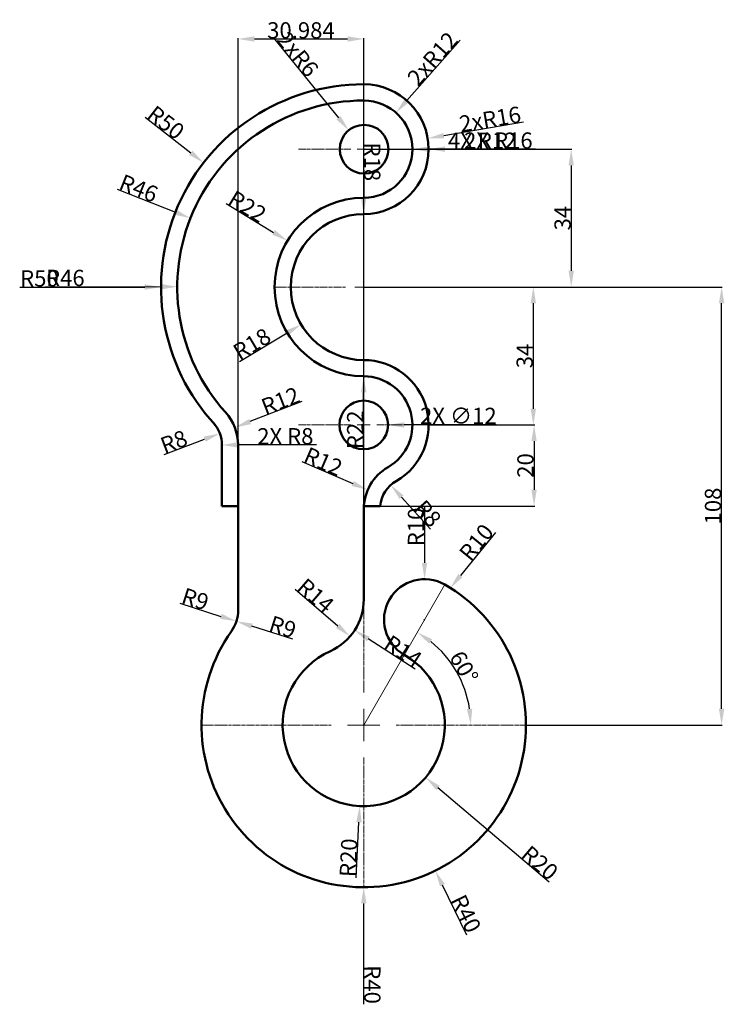
# Model space of a CAD drawing. Units: millimetres. Extents: x 64 to 238, y 47 to 290.
import ezdxf

# ---------------------------------------------------------------- set-up
doc = ezdxf.new("R2010")
doc.units = ezdxf.units.MM
doc.header["$MEASUREMENT"] = 0
doc.linetypes.add('CENTER2', pattern=[1.125, 0.75, -0.125, 0.125, -0.125])
for name, color, linetype, lineweight in [('M-CNTR', 4, 'CENTER2', 18), ('M-CONS', 8, 'Continuous', 13), ('M-DIMS', 2, 'Continuous', 25), ('M-OUTL', 7, 'Continuous', 50)]:
    doc.layers.add(name, color=color, linetype=linetype, lineweight=lineweight)
doc.styles.get("Standard").update_dxf_attribs({"font": 'arial.ttf'})
doc.dimstyles.get("Standard").update_dxf_attribs({"dimtxt": 4, "dimasz": 4, "dimexe": 0.18, "dimexo": 0.0625, "dimgap": 0.09, "dimtad": 1, "dimdec": 0, "dimzin": 0, "dimdsep": 46, "dimtxsty": 'Standard', "dimcen": 0.09, "dimclre": 251, "dimadec": 0, "dimazin": 0, "dimtfac": 1, "dimtdec": 0, "dimtofl": 0, "dimtmove": 0, "dimatfit": 3, "dimfxl": 1, "dimtolj": 1, "dimtzin": 0, "dimarcsym": 0})

# ---------------------------------------------------------------- blocks, each defined once
blk = doc.blocks.new('*U1')
at = {"layer": 'M-CNTR', "color": 0, "transparency": 16777216}
for p, q in [((0, 8), (0, 40.12)), ((-40.12, 0), (-8, 0)), ((8, 0), (40.12, 0)), ((0, -40.12), (0, -8))]:
    blk.add_line(p, q, dxfattribs=at)
at = {"layer": 'M-CNTR', "color": 0, "linetype": 'Continuous', "transparency": 16777216}
for p, q in [((0, -4), (0, 4)), ((-4, 0), (4, 0))]:
    blk.add_line(p, q, dxfattribs=at)
blk = doc.blocks.new('*U2')
at = {"layer": 'M-CNTR', "color": 0, "transparency": 16777216}
for p, q in [((0, 3.2), (0, 16.12)), ((-16.12, 0), (-3.2, 0)), ((3.2, 0), (16.12, 0)), ((0, -16.12), (0, -3.2))]:
    blk.add_line(p, q, dxfattribs=at)
at = {"layer": 'M-CNTR', "color": 0, "linetype": 'Continuous', "transparency": 16777216}
for p, q in [((-1.6, 0), (1.6, 0)), ((0, -1.6), (0, 1.6))]:
    blk.add_line(p, q, dxfattribs=at)
blk = doc.blocks.new('*U3')
at = {"layer": 'M-CNTR', "color": 0, "transparency": 16777216}
for p, q in [((0, 3.2), (0, 16.12)), ((-16.12, 0), (-3.2, 0)), ((3.2, 0), (16.12, 0)), ((0, -16.12), (0, -3.2))]:
    blk.add_line(p, q, dxfattribs=at)
at = {"layer": 'M-CNTR', "color": 0, "linetype": 'Continuous', "transparency": 16777216}
for p, q in [((-1.6, 0), (1.6, 0)), ((0, -1.6), (0, 1.6))]:
    blk.add_line(p, q, dxfattribs=at)
blk = doc.blocks.new('*D4')
at = {"layer": 'Defpoints', "color": 0, "transparency": 16777216}
for p in [(171.15, 223.67), (237.29, 223.67), (189.15, 115.67)]:
    blk.add_point(p, dxfattribs=at)
at = {"layer": 'M-DIMS', "color": 0, "lineweight": -2, "transparency": 16777216}
for p, q in [((171.21, 223.67), (237.47, 223.67)), ((237.29, 119.67), (237.29, 219.67)), ((189.21, 115.67), (237.47, 115.67))]:
    blk.add_line(p, q, dxfattribs=at)
at = {"layer": 'M-DIMS', "color": 0, "transparency": 16777216}
for points in [[(236.63, 219.67), (237.96, 219.67), (237.29, 223.67)], [(236.63, 119.67), (237.96, 119.67), (237.29, 115.67)]]:
    blk.add_solid(points, dxfattribs=at)
at = {"layer": 'M-DIMS', "color": 0, "transparency": 16777216, "insert": (235.16, 169.67), "char_height": 4, "attachment_point": 5, "rotation": 90}
blk.add_mtext('\\A1;108', dxfattribs=at)
blk = doc.blocks.new('*U5')
at = {"layer": 'M-CNTR', "color": 0, "transparency": 16777216}
for p, q in [((0, 4.4), (0, 22.12)), ((-22.12, 0), (-4.4, 0)), ((4.4, 0), (22.12, 0)), ((0, -22.12), (0, -4.4))]:
    blk.add_line(p, q, dxfattribs=at)
at = {"layer": 'M-CNTR', "color": 0, "linetype": 'Continuous', "transparency": 16777216}
for p, q in [((-2.2, 0), (2.2, 0)), ((0, -2.2), (0, 2.2))]:
    blk.add_line(p, q, dxfattribs=at)
blk = doc.blocks.new('*D6')
at = {"layer": 'Defpoints', "color": 0, "transparency": 16777216}
for p in [(171.15, 223.67), (165.03, 189.67), (190.85, 189.67)]:
    blk.add_point(p, dxfattribs=at)
at = {"layer": 'M-DIMS', "color": 0, "lineweight": -2, "transparency": 16777216}
for p, q in [((171.21, 223.67), (191.03, 223.67)), ((190.85, 219.67), (190.85, 193.67)), ((165.09, 189.67), (191.03, 189.67))]:
    blk.add_line(p, q, dxfattribs=at)
at = {"layer": 'M-DIMS', "color": 0, "transparency": 16777216}
for points in [[(190.19, 219.67), (191.52, 219.67), (190.85, 223.67)], [(190.19, 193.67), (191.52, 193.67), (190.85, 189.67)]]:
    blk.add_solid(points, dxfattribs=at)
at = {"layer": 'M-DIMS', "color": 0, "transparency": 16777216, "insert": (188.72, 206.67), "char_height": 4, "attachment_point": 5, "rotation": 90}
blk.add_mtext('\\A1;34', dxfattribs=at)
blk = doc.blocks.new('*D7')
at = {"layer": 'Defpoints', "color": 0, "transparency": 16777216}
for p in [(165.15, 189.67), (153.07, 169.67), (191.03, 169.67)]:
    blk.add_point(p, dxfattribs=at)
at = {"layer": 'M-DIMS', "color": 0, "lineweight": -2, "transparency": 16777216}
for p, q in [((165.21, 189.67), (191.21, 189.67)), ((191.03, 185.67), (191.03, 173.67)), ((153.13, 169.67), (191.21, 169.67))]:
    blk.add_line(p, q, dxfattribs=at)
at = {"layer": 'M-DIMS', "color": 0, "transparency": 16777216}
for points in [[(190.37, 185.67), (191.7, 185.67), (191.03, 189.67)], [(190.37, 173.67), (191.7, 173.67), (191.03, 169.67)]]:
    blk.add_solid(points, dxfattribs=at)
at = {"layer": 'M-DIMS', "color": 0, "transparency": 16777216, "insert": (188.9, 179.67), "char_height": 4, "attachment_point": 5, "rotation": 90}
blk.add_mtext('\\A1;20', dxfattribs=at)
blk = doc.blocks.new('*D8')
at = {"layer": 'Defpoints', "color": 0, "transparency": 16777216}
for p in [(109.52, 254.32), (149.03, 223.67)]:
    blk.add_point(p, dxfattribs=at)
at = {"layer": 'M-DIMS', "color": 0, "lineweight": -2, "transparency": 16777216}
for p, q in [((95.08, 265.53), (106.36, 256.77)), ((148.94, 223.67), (149.12, 223.67)), ((149.03, 223.58), (149.03, 223.76))]:
    blk.add_line(p, q, dxfattribs=at)
at = {"layer": 'M-DIMS', "color": 0, "transparency": 16777216}
blk.add_solid([(106.77, 257.3), (105.95, 256.24), (109.52, 254.32)], dxfattribs=at)
at = {"layer": 'M-DIMS', "color": 0, "transparency": 16777216, "insert": (100.23, 264.23), "char_height": 4, "attachment_point": 5, "rotation": 322.1908}
blk.add_mtext('\\A1;R50', dxfattribs=at)
blk = doc.blocks.new('*D9')
at = {"layer": 'Defpoints', "color": 0, "transparency": 16777216}
for p in [(106.28, 240.65), (149.03, 223.67)]:
    blk.add_point(p, dxfattribs=at)
at = {"layer": 'M-DIMS', "color": 0, "lineweight": -2, "transparency": 16777216}
for p, q in [((88.2, 247.83), (102.56, 242.13)), ((148.94, 223.67), (149.12, 223.67)), ((149.03, 223.58), (149.03, 223.76))]:
    blk.add_line(p, q, dxfattribs=at)
at = {"layer": 'M-DIMS', "color": 0, "transparency": 16777216}
blk.add_solid([(102.81, 242.75), (102.31, 241.51), (106.28, 240.65)], dxfattribs=at)
at = {"layer": 'M-DIMS', "color": 0, "transparency": 16777216, "insert": (93.51, 248.02), "char_height": 4, "attachment_point": 5, "rotation": 338.3318}
blk.add_mtext('\\A1;R46', dxfattribs=at)
blk = doc.blocks.new('*D10')
at = {"layer": 'Defpoints', "color": 0, "transparency": 16777216}
for p in [(130.22, 235.08), (149.03, 223.67)]:
    blk.add_point(p, dxfattribs=at)
at = {"layer": 'M-DIMS', "color": 0, "lineweight": -2, "transparency": 16777216}
for p, q in [((115.09, 244.26), (126.8, 237.15)), ((148.94, 223.67), (149.12, 223.67)), ((149.03, 223.58), (149.03, 223.76))]:
    blk.add_line(p, q, dxfattribs=at)
at = {"layer": 'M-DIMS', "color": 0, "transparency": 16777216}
blk.add_solid([(127.14, 237.72), (126.45, 236.58), (130.22, 235.08)], dxfattribs=at)
at = {"layer": 'M-DIMS', "color": 0, "transparency": 16777216, "insert": (120.32, 243.54), "char_height": 4, "attachment_point": 5, "rotation": 328.7559}
blk.add_mtext('\\A1;R22', dxfattribs=at)
blk = doc.blocks.new('*D11')
at = {"layer": 'Defpoints', "color": 0, "transparency": 16777216}
for p in [(149.03, 223.67), (133.58, 214.43)]:
    blk.add_point(p, dxfattribs=at)
at = {"layer": 'M-DIMS', "color": 0, "lineweight": -2, "transparency": 16777216}
for p, q in [((148.94, 223.67), (149.12, 223.67)), ((149.03, 223.58), (149.03, 223.76)), ((118.35, 205.32), (130.15, 212.37))]:
    blk.add_line(p, q, dxfattribs=at)
at = {"layer": 'M-DIMS', "color": 0, "transparency": 16777216}
blk.add_solid([(129.8, 212.95), (130.49, 211.8), (133.58, 214.43)], dxfattribs=at)
at = {"layer": 'M-DIMS', "color": 0, "transparency": 16777216, "insert": (121.44, 209.65), "char_height": 4, "attachment_point": 5, "rotation": 30.8847}
blk.add_mtext('\\A1;R18', dxfattribs=at)
blk = doc.blocks.new('*D12')
at = {"layer": 'Defpoints', "color": 0, "transparency": 16777216}
for p in [(113.52, 187.57), (106.04, 184.73)]:
    blk.add_point(p, dxfattribs=at)
at = {"layer": 'M-DIMS', "color": 0, "lineweight": -2, "transparency": 16777216}
blk.add_line((99.84, 182.36), (109.78, 186.15), dxfattribs=at)
at = {"layer": 'M-DIMS', "color": 0, "transparency": 16777216}
blk.add_solid([(109.54, 186.77), (110.02, 185.52), (113.52, 187.57)], dxfattribs=at)
at = {"layer": 'M-DIMS', "color": 0, "transparency": 16777216, "insert": (102.18, 185.54), "char_height": 4, "attachment_point": 5, "rotation": 20.8298}
blk.add_mtext('\\A1;R8', dxfattribs=at)
blk = doc.blocks.new('*D13')
at = {"layer": 'Defpoints', "color": 0, "transparency": 16777216}
for p in [(109.04, 143.99), (117.62, 141.26)]:
    blk.add_point(p, dxfattribs=at)
at = {"layer": 'M-DIMS', "color": 0, "lineweight": -2, "transparency": 16777216}
blk.add_line((103.67, 145.7), (113.81, 142.47), dxfattribs=at)
at = {"layer": 'M-DIMS', "color": 0, "transparency": 16777216}
blk.add_solid([(114.01, 143.11), (113.61, 141.84), (117.62, 141.26)], dxfattribs=at)
at = {"layer": 'M-DIMS', "color": 0, "transparency": 16777216, "insert": (107.48, 146.73), "char_height": 4, "attachment_point": 5, "rotation": 342.343}
blk.add_mtext('\\A1;R9', dxfattribs=at)
blk = doc.blocks.new('*D14')
at = {"layer": 'Defpoints', "color": 0, "transparency": 16777216}
for p in [(135.03, 146.65), (145.63, 137.51)]:
    blk.add_point(p, dxfattribs=at)
at = {"layer": 'M-DIMS', "color": 0, "lineweight": -2, "transparency": 16777216}
blk.add_line((132.12, 149.15), (142.6, 140.12), dxfattribs=at)
at = {"layer": 'M-DIMS', "color": 0, "transparency": 16777216}
blk.add_solid([(143.04, 140.63), (142.17, 139.62), (145.63, 137.51)], dxfattribs=at)
at = {"layer": 'M-DIMS', "color": 0, "transparency": 16777216, "insert": (137.17, 147.57), "char_height": 4, "attachment_point": 5, "rotation": 319.2597}
blk.add_mtext('\\A1;R14', dxfattribs=at)
blk = doc.blocks.new('*D15')
at = {"layer": 'Defpoints', "color": 0, "transparency": 16777216}
for p in [(150.01, 173.64), (161.03, 168.88)]:
    blk.add_point(p, dxfattribs=at)
at = {"layer": 'M-DIMS', "color": 0, "lineweight": -2, "transparency": 16777216}
for p, q in [((133.76, 180.66), (146.34, 175.23)), ((160.94, 168.88), (161.12, 168.88)), ((161.03, 168.79), (161.03, 168.97))]:
    blk.add_line(p, q, dxfattribs=at)
at = {"layer": 'M-DIMS', "color": 0, "transparency": 16777216}
blk.add_solid([(146.6, 175.84), (146.07, 174.61), (150.01, 173.64)], dxfattribs=at)
at = {"layer": 'M-DIMS', "color": 0, "transparency": 16777216, "insert": (139.05, 180.66), "char_height": 4, "attachment_point": 5, "rotation": 336.6403}
blk.add_mtext('\\A1;R12', dxfattribs=at)
blk = doc.blocks.new('*D16')
at = {"layer": 'Defpoints', "color": 0, "transparency": 16777216}
for p in [(155.68, 174.84), (161.03, 168.88)]:
    blk.add_point(p, dxfattribs=at)
at = {"layer": 'M-DIMS', "color": 0, "lineweight": -2, "transparency": 16777216}
blk.add_line((165.46, 163.94), (158.36, 171.86), dxfattribs=at)
at = {"layer": 'M-DIMS', "color": 0, "transparency": 16777216}
blk.add_solid([(158.85, 172.3), (157.86, 171.41), (155.68, 174.84)], dxfattribs=at)
at = {"layer": 'M-DIMS', "color": 0, "transparency": 16777216, "insert": (164.83, 167.84), "char_height": 4, "attachment_point": 5, "rotation": 311.9055}
blk.add_mtext('\\A1;R8', dxfattribs=at)
blk = doc.blocks.new('*D17')
at = {"layer": 'Defpoints', "color": 0, "transparency": 16777216}
for p in [(117.24, 189.04), (106.04, 184.73)]:
    blk.add_point(p, dxfattribs=at)
at = {"layer": 'M-DIMS', "color": 0, "lineweight": -2, "transparency": 16777216}
for p, q in [((133.75, 195.41), (120.97, 190.48)), ((105.95, 184.73), (106.13, 184.73)), ((106.04, 184.64), (106.04, 184.82))]:
    blk.add_line(p, q, dxfattribs=at)
at = {"layer": 'M-DIMS', "color": 0, "transparency": 16777216}
blk.add_solid([(120.73, 191.1), (121.21, 189.86), (117.24, 189.04)], dxfattribs=at)
at = {"layer": 'M-DIMS', "color": 0, "transparency": 16777216, "insert": (128.47, 195.62), "char_height": 4, "attachment_point": 5, "rotation": 21.0873}
blk.add_mtext('\\A1;R12', dxfattribs=at)
blk = doc.blocks.new('*D18')
at = {"layer": 'Defpoints', "color": 0, "transparency": 16777216}
for p in [(170.34, 149.4), (164.03, 141.65)]:
    blk.add_point(p, dxfattribs=at)
at = {"layer": 'M-DIMS', "color": 0, "lineweight": -2, "transparency": 16777216}
for p, q in [((181.52, 163.15), (172.86, 152.51)), ((163.94, 141.65), (164.12, 141.65)), ((164.03, 141.56), (164.03, 141.74))]:
    blk.add_line(p, q, dxfattribs=at)
blk.add_arc((164.03, 141.65), 10, 49.8391, 59.6419, dxfattribs=at)
at = {"layer": 'M-DIMS', "color": 0, "transparency": 16777216}
blk.add_solid([(172.34, 152.93), (173.38, 152.09), (170.34, 149.4)], dxfattribs=at)
at = {"layer": 'M-DIMS', "color": 0, "transparency": 16777216, "insert": (176.8, 160.73), "char_height": 4, "attachment_point": 5, "rotation": 50.8704}
blk.add_mtext('\\A1;R10', dxfattribs=at)
blk = doc.blocks.new('*D19')
at = {"layer": 'Defpoints', "color": 0, "transparency": 16777216}
for p in [(156.98, 266.65), (149.03, 257.67)]:
    blk.add_point(p, dxfattribs=at)
at = {"layer": 'M-DIMS', "color": 0, "lineweight": -2, "transparency": 16777216}
for p, q in [((172.81, 284.53), (159.63, 269.65)), ((148.94, 257.67), (149.12, 257.67)), ((149.03, 257.58), (149.03, 257.76))]:
    blk.add_line(p, q, dxfattribs=at)
at = {"layer": 'M-DIMS', "color": 0, "transparency": 16777216}
blk.add_solid([(159.13, 270.09), (160.13, 269.2), (156.98, 266.65)], dxfattribs=at)
at = {"layer": 'M-DIMS', "color": 0, "transparency": 16777216, "insert": (165.98, 279.97), "char_height": 4, "attachment_point": 5, "rotation": 48.4791}
blk.add_mtext('\\A1;2xR12', dxfattribs=at)
blk = doc.blocks.new('*D20')
at = {"layer": 'Defpoints', "color": 0, "transparency": 16777216}
for p in [(164.8, 260.32), (149.03, 257.67)]:
    blk.add_point(p, dxfattribs=at)
at = {"layer": 'M-DIMS', "color": 0, "lineweight": -2, "transparency": 16777216}
for p, q in [((188.39, 264.29), (168.75, 260.99)), ((148.94, 257.67), (149.12, 257.67)), ((149.03, 257.58), (149.03, 257.76))]:
    blk.add_line(p, q, dxfattribs=at)
at = {"layer": 'M-DIMS', "color": 0, "transparency": 16777216}
blk.add_solid([(168.64, 261.64), (168.86, 260.33), (164.8, 260.32)], dxfattribs=at)
at = {"layer": 'M-DIMS', "color": 0, "transparency": 16777216, "insert": (180.19, 265.07), "char_height": 4, "attachment_point": 5, "rotation": 9.5526}
blk.add_mtext('\\A1;2xR16', dxfattribs=at)
blk = doc.blocks.new('*D21')
at = {"layer": 'Defpoints', "color": 0, "transparency": 16777216}
for p in [(145.32, 262.31), (149.12, 257.67)]:
    blk.add_point(p, dxfattribs=at)
at = {"layer": 'M-DIMS', "color": 0, "lineweight": -2, "transparency": 16777216}
for p, q in [((127.06, 284.67), (142.79, 265.41)), ((149.03, 257.67), (149.21, 257.67)), ((149.12, 257.58), (149.12, 257.76))]:
    blk.add_line(p, q, dxfattribs=at)
at = {"layer": 'M-DIMS', "color": 0, "transparency": 16777216}
blk.add_solid([(143.31, 265.83), (142.27, 264.99), (145.32, 262.31)], dxfattribs=at)
at = {"layer": 'M-DIMS', "color": 0, "transparency": 16777216, "insert": (132.76, 281.06), "char_height": 4, "attachment_point": 5, "rotation": 309.2452}
blk.add_mtext('\\A1;2xR6', dxfattribs=at)
blk = doc.blocks.new('*D22')
at = {"layer": 'Defpoints', "color": 0, "transparency": 16777216}
for p in [(149.03, 115.67), (164.29, 102.74)]:
    blk.add_point(p, dxfattribs=at)
at = {"layer": 'M-DIMS', "color": 0, "lineweight": -2, "transparency": 16777216}
for p, q in [((148.94, 115.67), (149.12, 115.67)), ((149.03, 115.58), (149.03, 115.76)), ((194.77, 76.91), (167.34, 100.15))]:
    blk.add_line(p, q, dxfattribs=at)
at = {"layer": 'M-DIMS', "color": 0, "transparency": 16777216}
blk.add_solid([(167.77, 100.66), (166.91, 99.64), (164.29, 102.74)], dxfattribs=at)
at = {"layer": 'M-DIMS', "color": 0, "transparency": 16777216, "insert": (192.44, 81.68), "char_height": 4, "attachment_point": 5, "rotation": 319.7274}
blk.add_mtext('\\A1;R20', dxfattribs=at)
blk = doc.blocks.new('*D23')
at = {"layer": 'Defpoints', "color": 0, "transparency": 16777216}
for p in [(149.03, 115.67), (166.67, 79.77)]:
    blk.add_point(p, dxfattribs=at)
at = {"layer": 'M-DIMS', "color": 0, "lineweight": -2, "transparency": 16777216}
for p, q in [((148.94, 115.67), (149.12, 115.67)), ((149.03, 115.58), (149.03, 115.76)), ((174.49, 63.86), (168.43, 76.18))]:
    blk.add_line(p, q, dxfattribs=at)
at = {"layer": 'M-DIMS', "color": 0, "transparency": 16777216}
blk.add_solid([(169.03, 76.47), (167.84, 75.88), (166.67, 79.77)], dxfattribs=at)
at = {"layer": 'M-DIMS', "color": 0, "transparency": 16777216, "insert": (174.26, 69.16), "char_height": 4, "attachment_point": 5, "rotation": 296.1726}
blk.add_mtext('\\A1;R40', dxfattribs=at)
blk = doc.blocks.new('*D24')
at = {"layer": 'Defpoints', "color": 0, "transparency": 16777216}
for p in [(169.03, 150.31), (173.84, 124.7), (149.03, 115.67), (157.03, 115.67), (189.15, 115.67)]:
    blk.add_point(p, dxfattribs=at)
at = {"layer": 'M-DIMS', "color": 0, "lineweight": -2, "transparency": 16777216}
blk.add_arc((149.03, 115.67), 26.4, 8.6882, 51.3118, dxfattribs=at)
at = {"layer": 'M-DIMS', "color": 0, "transparency": 16777216}
for points in [[(165.16, 135.73), (165.91, 136.83), (162.23, 138.53)], [(175.79, 119.7), (174.46, 119.6), (175.43, 115.67)]]:
    blk.add_solid(points, dxfattribs=at)
at = {"layer": 'M-DIMS', "color": 0, "transparency": 16777216, "insert": (173.74, 129.93), "char_height": 4, "attachment_point": 5, "rotation": 300}
blk.add_mtext('\\A1;60°', dxfattribs=at)
blk = doc.blocks.new('*D25')
at = {"layer": 'Defpoints', "color": 0, "transparency": 16777216}
for p in [(149.03, 257.67), (149.03, 223.67), (200.2, 223.67)]:
    blk.add_point(p, dxfattribs=at)
at = {"layer": 'M-DIMS', "color": 251, "lineweight": -2, "transparency": 16777216}
for p, q in [((149.09, 257.67), (200.38, 257.67)), ((149.09, 223.67), (200.38, 223.67))]:
    blk.add_line(p, q, dxfattribs=at)
at = {"layer": 'M-DIMS', "color": 0, "lineweight": -2, "transparency": 16777216}
blk.add_line((200.2, 253.67), (200.2, 227.67), dxfattribs=at)
at = {"layer": 'M-DIMS', "color": 0, "transparency": 16777216}
for points in [[(199.53, 253.67), (200.86, 253.67), (200.2, 257.67)], [(199.53, 227.67), (200.86, 227.67), (200.2, 223.67)]]:
    blk.add_solid(points, dxfattribs=at)
at = {"layer": 'M-DIMS', "color": 0, "transparency": 16777216, "insert": (198.06, 240.67), "char_height": 4, "attachment_point": 5, "rotation": 90}
blk.add_mtext('\\A1;34', dxfattribs=at)
blk = doc.blocks.new('*D26')
at = {"layer": 'Defpoints', "color": 0, "transparency": 16777216}
for p in [(149.03, 284.84), (149.03, 146.65), (118.04, 143.99)]:
    blk.add_point(p, dxfattribs=at)
at = {"layer": 'M-DIMS', "color": 251, "lineweight": -2, "transparency": 16777216}
for p, q in [((118.04, 144.05), (118.04, 285.02)), ((149.03, 146.71), (149.03, 285.02))]:
    blk.add_line(p, q, dxfattribs=at)
at = {"layer": 'M-DIMS', "color": 0, "lineweight": -2, "transparency": 16777216}
blk.add_line((122.04, 284.84), (145.03, 284.84), dxfattribs=at)
at = {"layer": 'M-DIMS', "color": 0, "transparency": 16777216}
for points in [[(122.04, 285.5), (122.04, 284.17), (118.04, 284.84)], [(145.03, 285.5), (145.03, 284.17), (149.03, 284.84)]]:
    blk.add_solid(points, dxfattribs=at)
at = {"layer": 'M-DIMS', "color": 0, "transparency": 16777216, "insert": (133.53, 286.97), "char_height": 4, "attachment_point": 5}
blk.add_mtext('\\A1;30.984', dxfattribs=at)
blk = doc.blocks.new('*D27')
at = {"layer": 'Defpoints', "color": 0, "transparency": 16777216}
for p in [(99.03, 223.67), (149.03, 223.67)]:
    blk.add_point(p, dxfattribs=at)
at = {"layer": 'M-DIMS', "color": 0, "lineweight": -2, "transparency": 16777216}
blk.add_line((64.16, 223.67), (95.03, 223.67), dxfattribs=at)
at = {"layer": 'M-DIMS', "color": 251, "lineweight": -2, "transparency": 16777216}
for p, q in [((148.94, 223.67), (149.12, 223.67)), ((149.03, 223.58), (149.03, 223.76))]:
    blk.add_line(p, q, dxfattribs=at)
at = {"layer": 'M-DIMS', "color": 0, "transparency": 16777216}
blk.add_solid([(95.03, 224.34), (95.03, 223), (99.03, 223.67)], dxfattribs=at)
at = {"layer": 'M-DIMS', "color": 0, "transparency": 16777216, "insert": (69.03, 225.8), "char_height": 4, "attachment_point": 5, "rotation": 359.9954}
blk.add_mtext('\\A1;R50', dxfattribs=at)
blk = doc.blocks.new('*D28')
at = {"layer": 'Defpoints', "color": 0, "transparency": 16777216}
for p in [(103.03, 223.75), (149.03, 223.67)]:
    blk.add_point(p, dxfattribs=at)
at = {"layer": 'M-DIMS', "color": 0, "lineweight": -2, "transparency": 16777216}
blk.add_line((70.56, 223.81), (99.03, 223.76), dxfattribs=at)
at = {"layer": 'M-DIMS', "color": 251, "lineweight": -2, "transparency": 16777216}
for p, q in [((148.94, 223.67), (149.12, 223.67)), ((149.03, 223.58), (149.03, 223.76))]:
    blk.add_line(p, q, dxfattribs=at)
at = {"layer": 'M-DIMS', "color": 0, "transparency": 16777216}
blk.add_solid([(99.03, 224.42), (99.03, 223.09), (103.03, 223.75)], dxfattribs=at)
at = {"layer": 'M-DIMS', "color": 0, "transparency": 16777216, "insert": (75.43, 225.93), "char_height": 4, "attachment_point": 5, "rotation": 359.8953}
blk.add_mtext('\\A1;R46', dxfattribs=at)
blk = doc.blocks.new('*D29')
at = {"layer": 'Defpoints', "color": 0, "transparency": 16777216}
for p in [(149.03, 115.67), (149.03, 75.67)]:
    blk.add_point(p, dxfattribs=at)
at = {"layer": 'M-DIMS', "color": 251, "lineweight": -2, "transparency": 16777216}
for p, q in [((148.94, 115.67), (149.12, 115.67)), ((149.03, 115.58), (149.03, 115.76))]:
    blk.add_line(p, q, dxfattribs=at)
at = {"layer": 'M-DIMS', "color": 0, "lineweight": -2, "transparency": 16777216}
blk.add_line((149.03, 46.8), (149.03, 71.67), dxfattribs=at)
at = {"layer": 'M-DIMS', "color": 0, "transparency": 16777216}
blk.add_solid([(149.7, 71.67), (148.36, 71.67), (149.03, 75.67)], dxfattribs=at)
at = {"layer": 'M-DIMS', "color": 0, "transparency": 16777216, "insert": (151.16, 51.67), "char_height": 4, "attachment_point": 5, "rotation": 270.0048}
blk.add_mtext('\\A1;R40', dxfattribs=at)
blk = doc.blocks.new('*D30')
at = {"layer": 'Defpoints', "color": 0, "transparency": 16777216}
for p in [(149.03, 223.67), (149.01, 201.67)]:
    blk.add_point(p, dxfattribs=at)
at = {"layer": 'M-DIMS', "color": 251, "lineweight": -2, "transparency": 16777216}
for p, q in [((148.94, 223.67), (149.12, 223.67)), ((149.03, 223.58), (149.03, 223.76))]:
    blk.add_line(p, q, dxfattribs=at)
at = {"layer": 'M-DIMS', "color": 0, "lineweight": -2, "transparency": 16777216}
blk.add_line((148.99, 183.62), (149, 197.67), dxfattribs=at)
at = {"layer": 'M-DIMS', "color": 0, "transparency": 16777216}
blk.add_solid([(148.34, 197.67), (149.67, 197.67), (149.01, 201.67)], dxfattribs=at)
at = {"layer": 'M-DIMS', "color": 0, "transparency": 16777216, "insert": (146.9, 188.47), "char_height": 4, "attachment_point": 5, "rotation": 89.9489}
blk.add_mtext('\\A1;R22', dxfattribs=at)
blk = doc.blocks.new('*D31')
at = {"layer": 'Defpoints', "color": 0, "transparency": 16777216}
for p in [(149.03, 115.67), (148.03, 95.69)]:
    blk.add_point(p, dxfattribs=at)
at = {"layer": 'M-DIMS', "color": 251, "lineweight": -2, "transparency": 16777216}
for p, q in [((148.94, 115.67), (149.12, 115.67)), ((149.03, 115.58), (149.03, 115.76))]:
    blk.add_line(p, q, dxfattribs=at)
at = {"layer": 'M-DIMS', "color": 0, "lineweight": -2, "transparency": 16777216}
blk.add_line((147.16, 77.99), (147.84, 91.7), dxfattribs=at)
at = {"layer": 'M-DIMS', "color": 0, "transparency": 16777216}
blk.add_solid([(147.17, 91.73), (148.5, 91.66), (148.03, 95.69)], dxfattribs=at)
at = {"layer": 'M-DIMS', "color": 0, "transparency": 16777216, "insert": (145.27, 82.95), "char_height": 4, "attachment_point": 5, "rotation": 87.158}
blk.add_mtext('\\A1;R20', dxfattribs=at)
blk = doc.blocks.new('*D32')
at = {"layer": 'Defpoints', "color": 0, "transparency": 16777216}
for p in [(149.01, 241.67), (149.03, 223.67)]:
    blk.add_point(p, dxfattribs=at)
at = {"layer": 'M-DIMS', "color": 0, "lineweight": -2, "transparency": 16777216}
blk.add_line((148.99, 259.41), (149.01, 245.67), dxfattribs=at)
at = {"layer": 'M-DIMS', "color": 251, "lineweight": -2, "transparency": 16777216}
for p, q in [((148.94, 223.67), (149.12, 223.67)), ((149.03, 223.58), (149.03, 223.76))]:
    blk.add_line(p, q, dxfattribs=at)
at = {"layer": 'M-DIMS', "color": 0, "transparency": 16777216}
blk.add_solid([(149.67, 245.67), (148.34, 245.67), (149.01, 241.67)], dxfattribs=at)
at = {"layer": 'M-DIMS', "color": 0, "transparency": 16777216, "insert": (151.13, 254.54), "char_height": 4, "attachment_point": 5, "rotation": 270.0529}
blk.add_mtext('\\A1;R18', dxfattribs=at)
blk = doc.blocks.new('*D33')
at = {"layer": 'Defpoints', "color": 0, "transparency": 16777216}
for p in [(149.03, 257.67), (165.03, 257.67)]:
    blk.add_point(p, dxfattribs=at)
at = {"layer": 'M-DIMS', "color": 251, "lineweight": -2, "transparency": 16777216}
for p, q in [((148.94, 257.67), (149.12, 257.67)), ((149.03, 257.58), (149.03, 257.76))]:
    blk.add_line(p, q, dxfattribs=at)
at = {"layer": 'M-DIMS', "color": 0, "lineweight": -2, "transparency": 16777216}
blk.add_line((191.42, 257.67), (169.03, 257.67), dxfattribs=at)
at = {"layer": 'M-DIMS', "color": 0, "transparency": 16777216}
blk.add_solid([(169.03, 258.33), (169.03, 257), (165.03, 257.67)], dxfattribs=at)
at = {"layer": 'M-DIMS', "color": 0, "transparency": 16777216, "insert": (182.23, 259.8), "char_height": 4, "attachment_point": 5, "rotation": 0.0001}
blk.add_mtext('\\A1;2X R16', dxfattribs=at)
blk = doc.blocks.new('*D34')
at = {"layer": 'Defpoints', "color": 0, "transparency": 16777216}
for p in [(135.03, 146.65), (146.79, 139.06)]:
    blk.add_point(p, dxfattribs=at)
at = {"layer": 'M-DIMS', "color": 251, "lineweight": -2, "transparency": 16777216}
for p, q in [((134.94, 146.65), (135.12, 146.65)), ((135.03, 146.56), (135.03, 146.74))]:
    blk.add_line(p, q, dxfattribs=at)
at = {"layer": 'M-DIMS', "color": 0, "lineweight": -2, "transparency": 16777216}
blk.add_line((161.68, 129.45), (150.15, 136.89), dxfattribs=at)
at = {"layer": 'M-DIMS', "color": 0, "transparency": 16777216}
blk.add_solid([(150.51, 137.45), (149.79, 136.33), (146.79, 139.06)], dxfattribs=at)
at = {"layer": 'M-DIMS', "color": 0, "transparency": 16777216, "insert": (158.73, 133.84), "char_height": 4, "attachment_point": 5, "rotation": 327.157}
blk.add_mtext('\\A1;R14', dxfattribs=at)
blk = doc.blocks.new('*D35')
at = {"layer": 'Defpoints', "color": 0, "transparency": 16777216}
for p in [(149.03, 257.67), (161.03, 257.67)]:
    blk.add_point(p, dxfattribs=at)
at = {"layer": 'M-DIMS', "color": 251, "lineweight": -2, "transparency": 16777216}
for p, q in [((148.94, 257.67), (149.12, 257.67)), ((149.03, 257.58), (149.03, 257.76))]:
    blk.add_line(p, q, dxfattribs=at)
at = {"layer": 'M-DIMS', "color": 0, "lineweight": -2, "transparency": 16777216}
blk.add_line((187.48, 257.67), (165.03, 257.67), dxfattribs=at)
at = {"layer": 'M-DIMS', "color": 0, "transparency": 16777216}
blk.add_solid([(165.03, 258.33), (165.03, 257), (161.03, 257.67)], dxfattribs=at)
at = {"layer": 'M-DIMS', "color": 0, "transparency": 16777216, "insert": (178.25, 259.77), "char_height": 4, "attachment_point": 5, "rotation": 0.0001}
blk.add_mtext('\\A1;4X R12', dxfattribs=at)
blk = doc.blocks.new('*D36')
at = {"layer": 'Defpoints', "color": 0, "transparency": 16777216}
for p in [(164.03, 151.65), (164.03, 141.65)]:
    blk.add_point(p, dxfattribs=at)
at = {"layer": 'M-DIMS', "color": 0, "lineweight": -2, "transparency": 16777216}
blk.add_line((164.03, 169.37), (164.03, 155.65), dxfattribs=at)
at = {"layer": 'M-DIMS', "color": 251, "lineweight": -2, "transparency": 16777216}
for p, q in [((163.94, 141.65), (164.12, 141.65)), ((164.03, 141.56), (164.03, 141.74))]:
    blk.add_line(p, q, dxfattribs=at)
at = {"layer": 'M-DIMS', "color": 0, "transparency": 16777216}
blk.add_solid([(163.36, 155.65), (164.69, 155.65), (164.03, 151.65)], dxfattribs=at)
at = {"layer": 'M-DIMS', "color": 0, "transparency": 16777216, "insert": (161.9, 164.51), "char_height": 4, "attachment_point": 5, "rotation": 89.9979}
blk.add_mtext('\\A1;R10', dxfattribs=at)
blk = doc.blocks.new('*D37')
at = {"layer": 'Defpoints', "color": 0, "transparency": 16777216}
for p in [(109.04, 143.99), (117.62, 141.26)]:
    blk.add_point(p, dxfattribs=at)
at = {"layer": 'M-DIMS', "color": 251, "lineweight": -2, "transparency": 16777216}
for p, q in [((108.95, 143.99), (109.13, 143.99)), ((109.04, 143.9), (109.04, 144.08))]:
    blk.add_line(p, q, dxfattribs=at)
at = {"layer": 'M-DIMS', "color": 0, "lineweight": -2, "transparency": 16777216}
blk.add_line((131.57, 136.82), (121.43, 140.05), dxfattribs=at)
at = {"layer": 'M-DIMS', "color": 0, "transparency": 16777216}
blk.add_solid([(121.63, 140.68), (121.23, 139.41), (117.62, 141.26)], dxfattribs=at)
at = {"layer": 'M-DIMS', "color": 0, "transparency": 16777216, "insert": (129.05, 139.86), "char_height": 4, "attachment_point": 5, "rotation": 342.3444}
blk.add_mtext('\\A1;R9', dxfattribs=at)
blk = doc.blocks.new('*D38')
at = {"layer": 'Defpoints', "color": 0, "transparency": 16777216}
for p in [(106.04, 184.73), (114.04, 184.73)]:
    blk.add_point(p, dxfattribs=at)
at = {"layer": 'M-DIMS', "color": 251, "lineweight": -2, "transparency": 16777216}
for p, q in [((105.95, 184.73), (106.13, 184.73)), ((106.04, 184.64), (106.04, 184.82))]:
    blk.add_line(p, q, dxfattribs=at)
at = {"layer": 'M-DIMS', "color": 0, "lineweight": -2, "transparency": 16777216}
blk.add_line((137.34, 184.76), (118.04, 184.74), dxfattribs=at)
at = {"layer": 'M-DIMS', "color": 0, "transparency": 16777216}
blk.add_solid([(118.04, 185.4), (118.04, 184.07), (114.04, 184.73)], dxfattribs=at)
at = {"layer": 'M-DIMS', "color": 0, "transparency": 16777216, "insert": (129.69, 186.88), "char_height": 4, "attachment_point": 5, "rotation": 0.0562}
blk.add_mtext('\\A1;2X R8', dxfattribs=at)
blk = doc.blocks.new('*D39')
at = {"layer": 'Defpoints', "color": 0, "transparency": 16777216}
for p in [(143.03, 189.67), (155.03, 189.67)]:
    blk.add_point(p, dxfattribs=at)
at = {"layer": 'M-DIMS', "color": 251, "lineweight": -2, "transparency": 16777216}
for p, q in [((148.94, 189.67), (149.12, 189.67)), ((149.03, 189.58), (149.03, 189.76))]:
    blk.add_line(p, q, dxfattribs=at)
at = {"layer": 'M-DIMS', "color": 0, "lineweight": -2, "transparency": 16777216}
blk.add_line((181.7, 189.67), (159.03, 189.67), dxfattribs=at)
at = {"layer": 'M-DIMS', "color": 0, "transparency": 16777216}
blk.add_solid([(159.03, 190.33), (159.03, 189), (155.03, 189.67)], dxfattribs=at)
at = {"layer": 'M-DIMS', "color": 0, "transparency": 16777216, "insert": (172.36, 191.91), "char_height": 4, "attachment_point": 5, "rotation": 0.0003}
blk.add_mtext('\\A1;2X ∅12', dxfattribs=at)

msp = doc.modelspace()

# ---------------------------------------------------------------- linework, layer by layer
at = {"layer": 'M-CONS'}
msp.add_line((149.0266, 115.666), (169.0266, 150.307), dxfattribs=at)
at = {"layer": 'M-OUTL'}
for p, q in [((114.0428, 184.7252), (114.0428, 169.666)), ((118.0428, 184.7252), (118.0428, 143.9907)), ((114.0428, 169.666), (118.0428, 169.666)), ((149.0266, 146.6498), (149.0266, 168.8814)), ((153.0652, 169.666), (149.0523, 169.666)), ((149.0523, 169.666), (153.0652, 169.666))]:
    msp.add_line(p, q, dxfattribs=at)
for centre in [(149.1166, 257.666), (149.0266, 189.666)]:
    msp.add_circle(centre, 6, dxfattribs=at)
for centre, radius, start, end in [((149.0266, 223.666), 50, 90, 222.843643), ((149.0266, 257.666), 16, 270, 90), ((149.0266, 223.666), 46, 90, 222.174699), ((149.0266, 257.666), 12, 270, 90), ((149.0266, 223.666), 22, 90, 270), ((149.0266, 223.666), 18, 90, 270), ((149.0266, 189.666), 16, 300, 90), ((149.0266, 189.666), 12, 300, 90), ((106.0428, 184.7252), 12, 0, 42.174699), ((106.0428, 184.7252), 8, 0, 42.174699), ((161.0266, 168.8814), 12, 120, 180), ((161.0266, 168.8814), 8, 120, 174.371599), ((164.0266, 141.6467), 10, 60, 240), ((149.0266, 115.666), 40, 144.68609, 60), ((135.0266, 146.6498), 14, 294.315739, 0), ((109.0428, 143.9907), 9, 324.68609, 0), ((149.0266, 115.666), 20, 114.315739, 60)]:
    msp.add_arc(centre, radius, start, end, dxfattribs=at)

# ---------------------------------------------------------------- block references
at = {"layer": 'M-CNTR'}
for name, p in [('*U3', (149.0266, 257.666)), ('*U5', (149.0266, 223.666)), ('*U2', (149.0266, 189.666)), ('*U1', (149.0266, 115.666))]:
    msp.add_blockref(name, p, dxfattribs=at)

# ---------------------------------------------------------------- dimensions: what is measured, and where the dimension line sits
at = {"layer": 'M-DIMS'}
dim = msp.add_linear_dim(base=(149.0266, 284.836), p1=(118.0428, 143.9907), p2=(149.0266, 146.6498), dimstyle='Standard', override={"dimdec": 3, "dimlfac": 1, "dimrnd": 0, "dimzin": 0, "dimdsep": 46, "dimlunit": 2}, dxfattribs=at)
dim.commit()
dim.dimension.update_dxf_attribs({"geometry": '*D26', "text_midpoint": (133.5347, 286.9696)})
dim = msp.add_radius_dim(center=(149.1166, 257.666), mpoint=(145.3208, 262.3126), text='2x<>', dimstyle='Standard', override={"dimclrd": 0, "dimclre": 0, "dimclrt": 0}, dxfattribs=at)
dim.commit()
dim.dimension.update_dxf_attribs({"geometry": '*D21', "text_midpoint": (131.1106, 279.708), "dimtype": 164})
for center, mpoint, text, override, picture, middle in [((149.0266, 257.666), (156.9813, 266.6505), '2x<>', {"dimclrd": 0, "dimclre": 0, "dimclrt": 0}, '*D19', (165.9751, 279.9738)), ((149.0266, 257.666), (164.8048, 260.3212), '2x<>', {"dimclrd": 0, "dimclre": 0, "dimclrt": 0}, '*D20', (180.186, 265.0719)), ((149.0266, 257.666), (165.0266, 257.666), '2X <>', {"dimdec": 0, "dimlfac": 1, "dimrnd": 0, "dimzin": 0, "dimdsep": 46, "dimlunit": 2}, '*D33', (182.2258, 259.7983)), ((149.0266, 257.666), (161.0266, 257.666), '4X <>', {"dimdec": 0, "dimlfac": 1, "dimrnd": 0, "dimzin": 0, "dimdsep": 46, "dimlunit": 2}, '*D35', (178.2531, 259.7656)), ((106.0428, 184.7252), (114.0428, 184.733), '2X <>', {"dimdec": 0, "dimlfac": 1, "dimrnd": 0, "dimzin": 0, "dimdsep": 46, "dimlunit": 2}, '*D38', (129.6914, 186.8806))]:
    dim = msp.add_radius_dim(center=center, mpoint=mpoint, text=text, dimstyle='Standard', override=override, dxfattribs=at)
    dim.commit()
    dim.dimension.update_dxf_attribs({"geometry": picture, "text_midpoint": middle})
for center, mpoint, override, picture, middle in [((149.0266, 223.666), (109.5238, 254.3177), {"dimclrd": 0, "dimclre": 0, "dimclrt": 0}, '*D8', (98.9192, 262.5462)), ((149.0266, 223.666), (106.2771, 240.6506), {"dimclrd": 0, "dimclre": 0, "dimclrt": 0}, '*D9', (92.7206, 246.0367)), ((149.0266, 223.666), (99.0266, 223.67), {"dimdec": 0, "dimlfac": 1, "dimrnd": 0, "dimzin": 0, "dimdsep": 46, "dimlunit": 2}, '*D27', (69.0266, 223.6724)), ((149.0266, 223.666), (103.0267, 223.75), {"dimdec": 0, "dimlfac": 1, "dimrnd": 0, "dimzin": 0, "dimdsep": 46, "dimlunit": 2}, '*D28', (75.4268, 223.8004)), ((149.0266, 223.666), (149.007, 201.666), {"dimdec": 0, "dimlfac": 1, "dimrnd": 0, "dimzin": 0, "dimdsep": 46, "dimlunit": 2}, '*D30', (148.9952, 188.466)), ((106.0428, 184.7252), (113.5199, 187.5699), {"dimclrd": 0, "dimclre": 0, "dimclrt": 0}, '*D12', (102.9405, 183.5449)), ((161.0266, 168.8814), (155.6834, 174.8353), {"dimclrd": 0, "dimclre": 0, "dimclrt": 0}, '*D16', (163.2435, 166.4111)), ((135.0266, 146.6498), (145.6341, 137.513), {"dimclrd": 0, "dimclre": 0, "dimclrt": 0}, '*D14', (135.8035, 145.9807)), ((109.0428, 143.9907), (117.6188, 141.2608), {"dimclrd": 0, "dimclre": 0, "dimclrt": 0}, '*D13', (106.8328, 144.6942)), ((149.0266, 115.666), (149.03, 75.666), {"dimdec": 0, "dimlfac": 1, "dimrnd": 0, "dimzin": 0, "dimdsep": 46, "dimlunit": 2}, '*D29', (149.032, 51.666)), ((149.0266, 115.666), (164.2862, 102.7375), {"dimclrd": 0, "dimclre": 0, "dimclrt": 0}, '*D22', (191.0639, 80.0504))]:
    dim = msp.add_radius_dim(center=center, mpoint=mpoint, dimstyle='Standard', override=override, dxfattribs=at)
    dim.commit()
    dim.dimension.update_dxf_attribs({"geometry": picture, "text_midpoint": middle, "dimtype": 164})
for center, mpoint, override, picture, middle in [((149.0266, 223.666), (149.01, 241.666), {"dimdec": 0, "dimlfac": 1, "dimrnd": 0, "dimzin": 0, "dimdsep": 46, "dimlunit": 2}, '*D32', (151.1304, 254.541)), ((149.0266, 223.666), (130.2174, 235.077), {"dimclrd": 0, "dimclre": 0, "dimclrt": 0}, '*D10', (120.3207, 243.5353)), ((149.0266, 223.666), (133.579, 214.4264), {"dimclrd": 0, "dimclre": 0, "dimclrt": 0}, '*D11', (121.4368, 209.6484)), ((106.0428, 184.7252), (117.2392, 189.0426), {"dimclrd": 0, "dimclre": 0, "dimclrt": 0}, '*D17', (128.4724, 195.6231)), ((161.0266, 168.8814), (150.0102, 173.6394), {"dimclrd": 0, "dimclre": 0, "dimclrt": 0}, '*D15', (139.0468, 180.6601)), ((164.0266, 141.6467), (164.027, 151.6467), {"dimdec": 0, "dimlfac": 1, "dimrnd": 0, "dimzin": 0, "dimdsep": 46, "dimlunit": 2}, '*D36', (161.8952, 164.509)), ((164.0266, 141.6467), (170.3374, 149.4039), {"dimclrd": 0, "dimclre": 0, "dimclrt": 0}, '*D18', (176.8003, 160.727)), ((135.0266, 146.6498), (146.7889, 139.0571), {"dimdec": 0, "dimlfac": 1, "dimrnd": 0, "dimzin": 0, "dimdsep": 46, "dimlunit": 2}, '*D34', (158.7319, 133.845)), ((109.0428, 143.9907), (117.6188, 141.2611), {"dimdec": 0, "dimlfac": 1, "dimrnd": 0, "dimzin": 0, "dimdsep": 46, "dimlunit": 2}, '*D37', (129.0516, 139.8599)), ((149.0266, 115.666), (148.035, 95.6906), {"dimdec": 0, "dimlfac": 1, "dimrnd": 0, "dimzin": 0, "dimdsep": 46, "dimlunit": 2}, '*D31', (145.2676, 82.9499)), ((149.0266, 115.666), (166.6697, 79.7672), {"dimclrd": 0, "dimclre": 0, "dimclrt": 0}, '*D23', (174.2566, 69.1643))]:
    dim = msp.add_radius_dim(center=center, mpoint=mpoint, dimstyle='Standard', override=override, dxfattribs=at)
    dim.commit()
    dim.dimension.update_dxf_attribs({"geometry": picture, "text_midpoint": middle})
for base, p1, p2, override, picture, middle in [((200.1966, 223.666), (149.0266, 257.666), (149.0266, 223.666), {"dimdec": 0, "dimlfac": 1, "dimrnd": 0, "dimzin": 0, "dimdsep": 46, "dimlunit": 2}, '*D25', (198.063, 240.666)), ((190.854, 189.666), (171.1466, 223.666), (165.0266, 189.666), {"dimclrd": 0, "dimclre": 0, "dimclrt": 0}, '*D6', (188.7203, 206.666)), ((237.2927, 223.666), (189.1466, 115.666), (171.1466, 223.666), {"dimclrd": 0, "dimclre": 0, "dimclrt": 0}, '*D4', (235.1605, 169.666)), ((191.034, 169.666), (165.1466, 189.666), (153.0652, 169.666), {"dimclrd": 0, "dimclre": 0, "dimclrt": 0}, '*D7', (188.9017, 179.666))]:
    dim = msp.add_linear_dim(base=base, p1=p1, p2=p2, angle=90, dimstyle='Standard', override=override, dxfattribs=at)
    dim.commit()
    dim.dimension.update_dxf_attribs({"geometry": picture, "text_midpoint": middle})
dim = msp.add_diameter_dim_2p(p1=(143.0266, 189.6659), p2=(155.0266, 189.666), text='2X <>', dimstyle='Standard', override={"dimdec": 0, "dimlfac": 1, "dimrnd": 0, "dimzin": 0, "dimdsep": 46, "dimlunit": 2}, dxfattribs=at)
dim.commit()
dim.dimension.update_dxf_attribs({"geometry": '*D39', "text_midpoint": (172.3622, 189.6661), "dimtype": 163})
dim = msp.add_angular_dim_2l(base=(173.8383, 124.6967), line1=((157.0266, 115.666), (189.1466, 115.666)), line2=((149.0266, 115.666), (169.0266, 150.307)), dimstyle='Standard', override={"dimclrd": 0, "dimclre": 0, "dimclrt": 0}, dxfattribs=at)
dim.commit()
dim.dimension.update_dxf_attribs({"geometry": '*D24', "text_midpoint": (171.8932, 128.868), "dimtype": 162})

doc.saveas('drawing.dxf')
